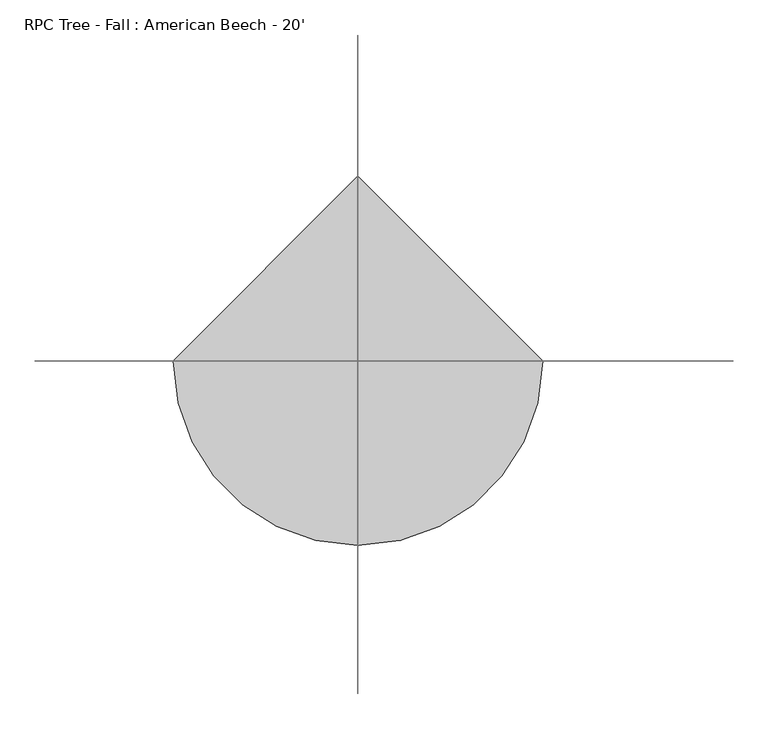
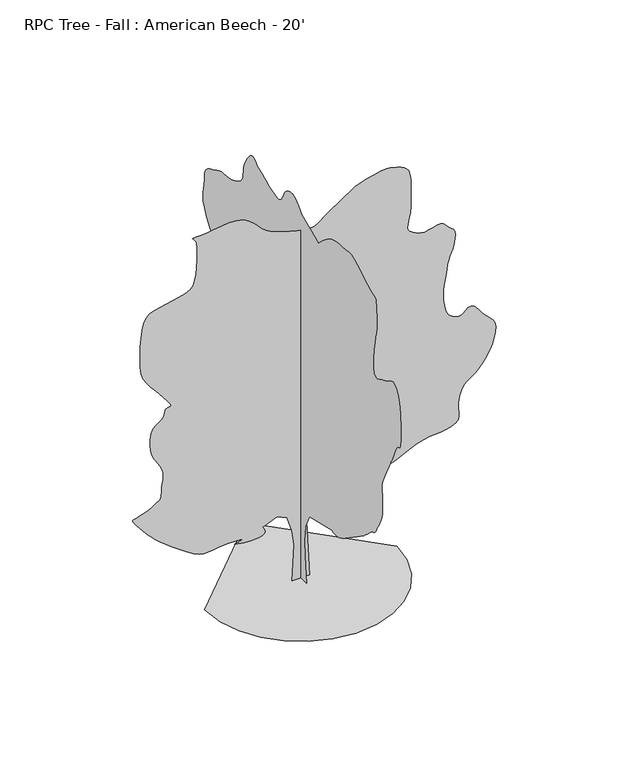
"""IFC4 building model written with IfcOpenShell, lengths in millimetres: geographic element geometry, RPC Tree - Fall : American Beech - 20'."""

from ifc_helpers import new_model, si_unit, origin, place, context, project, spatial, triangles, source, transform, mapped, element, save


def rpc_tree_fall_american_beech_20_7ed35302(model_context):
    return source(origin(), model_context, "Body", "Tessellation", [
        triangles([(0.0003461, 47.8998015, 0.0), (0.0003461, -52.4491741, 0.0), (0.0003461, -39.0692677, 147.1785164), (0.0003461, -35.7244046, 230.8023728), (0.0003461, -42.4141353, 314.4262293), (0.0003461, -82.5537637, 391.3603415), (0.0003461, -286.5960421, 441.5346408), (0.0003461, -297.4800798, 437.3999004), (0.0003461, -309.1526776, 434.2599395), (0.0003461, -322.4059021, 433.1087016), (0.0003461, -338.0291854, 434.9427103), (0.0003461, -356.8111058, 440.7550009), (0.0003461, -379.5428578, 451.5403527), (0.0003461, -407.0147638, 468.2944536), (0.0003461, -517.3983968, 545.2285658), (0.0003461, -533.0021682, 556.1997348), (0.0003461, -548.4298602, 566.6437194), (0.0003461, -563.9162696, 577.2637107), (0.0003461, -579.6951393, 588.7620641), (0.0003461, -596.0002851, 601.8392455), (0.0003461, -613.0664309, 617.1985188), (0.0003461, -631.1273924, 635.5421665), (0.0003461, -646.779126, 650.3066723), (0.0003461, -657.6329693, 656.9973249), (0.0003461, -665.4445564, 659.4154186), (0.0003461, -671.9689402, 661.365881), (0.0003461, -678.9609552, 666.6518229), (0.0003461, -688.1763084, 679.0756285), (0.0003461, -701.3708519, 702.4421528), (0.0003461, -715.7362541, 729.1227917), (0.0003461, -727.4097422, 750.8313503), (0.0003461, -736.5664507, 770.3741982), (0.0003461, -743.3832584, 790.5616287), (0.0003461, -748.0354454, 814.2001568), (0.0003461, -750.6971289, 844.0999306), (0.0003461, -751.5460596, 883.0692816), (0.0003461, -749.8880939, 918.7111467), (0.0003461, -746.4752209, 940.9005627), (0.0003461, -743.6463964, 955.8269045), (0.0003461, -743.7442102, 969.7041824), (0.0003461, -749.1075457, 988.7288206), (0.0003461, -762.0780476, 1019.1148293), (0.0003461, -784.9956167, 1067.040901), (0.0003461, -808.0492241, 1113.6867456), (0.0003461, -821.9754089, 1140.7834929), (0.0003461, -829.9328447, 1155.4253317), (0.0003461, -835.081949, 1164.679854), (0.0003461, -840.5821947, 1175.6323105), (0.0003461, -849.5930546, 1195.3592314), (0.0003461, -865.2741468, 1230.94594), (0.0003461, -882.983967, 1263.376664), (0.0003461, -896.3616388, 1275.8049751), (0.0003461, -905.9984053, 1278.5164375), (0.0003461, -912.4703213, 1281.8146374), (0.0003461, -916.3730627, 1295.9941498), (0.0003461, -918.2844286, 1331.3496952), (0.0003461, -918.7911564, 1398.1935802), (0.0003461, -915.3773386, 1473.7498695), (0.0003461, -906.2295685, 1530.0057381), (0.0003461, -892.9922951, 1569.3440346), (0.0003461, -877.2890385, 1594.1739143), (0.0003461, -860.7686806, 1606.8865105), (0.0003461, -845.0680401, 1609.8914143), (0.0003461, -831.8246624, 1605.5797588), (0.0003461, -820.3467293, 1598.43223), (0.0003461, -808.8101515, 1591.4001011), (0.0003461, -797.1562843, 1584.6082191), (0.0003461, -785.3272099, 1578.1541073), (0.0003461, -773.263484, 1572.179908), (0.0003461, -760.9081335, 1566.7837257), (0.0003461, -748.2007696, 1562.0986919), (0.0003461, -733.7483088, 1555.2800674), (0.0003461, -717.3649338, 1546.4701401), (0.0003461, -700.8054794, 1540.238253), (0.0003461, -685.8267426, 1541.1450291), (0.0003461, -674.1826132, 1553.7598114), (0.0003461, -667.6288708, 1582.6346478), (0.0003461, -667.9213675, 1632.3385906), (0.0003461, -673.2757645, 1686.7987839), (0.0003461, -680.0340002, 1729.2575294), (0.0003461, -687.1433046, 1763.2884464), (0.0003461, -693.5503263, 1792.4654446), (0.0003461, -698.2025133, 1820.3622883), (0.0003461, -700.0454241, 1850.5350105), (0.0003461, -698.0264339, 1886.5572304), (0.0003461, -695.2279129, 1921.1216904), (0.0003461, -694.0668646, 1945.9691563), (0.0003461, -692.4969023, 1963.2691177), (0.0003461, -688.4696772, 1975.1817627), (0.0003461, -679.9361864, 1983.8851559), (0.0003461, -664.8498253, 1991.5304741), (0.0003461, -641.1623903, 2000.287207), (0.0003461, -611.9542894, 2013.186565), (0.0003461, -581.9869689, 2030.1842194), (0.0003461, -551.7254076, 2048.8265408), (0.0003461, -521.640725, 2066.6421684), (0.0003461, -492.1996805, 2081.1773277), (0.0003461, -463.8699054, 2089.9874004), (0.0003461, -437.1198667, 2090.6007351), (0.0003461, -410.9841436, 2087.1692585), (0.0003461, -384.4972429, 2084.8489059), (0.0003461, -358.1277042, 2082.6975838), (0.0003461, -332.3431226, 2079.7904938), (0.0003461, -307.6120377, 2075.194408), (0.0003461, -284.40199, 2067.9579311), (0.0003461, -263.1815556, 2057.1476898), (0.0003461, -244.2822913, 2044.4438141), (0.0003461, -227.4890576, 2032.0867195), (0.0003461, -212.4516034, 2020.022921), (0.0003461, -198.8178971, 2008.1992241), (0.0003461, -186.2376512, 1996.5444122), (0.0003461, -174.3597061, 1985.005291), (0.0003461, -162.8329206, 1973.5282299), (0.0003461, -5.6196759, 2040.4256001), (0.0003461, 7.9941966, 2055.3518692), (0.0003461, 21.5788041, 2069.5581242), (0.0003461, 35.1049498, 2082.2885971), (0.0003461, 48.5432624, 2092.8321396), (0.0003461, 61.8645832, 2100.4508606), (0.0003461, 75.0396602, 2104.4068691), (0.0003461, 88.0391665, 2103.980151), (0.0003461, 100.5219802, 2100.8509815), (0.0003461, 112.1269949, 2096.9570332), (0.0003461, 122.7958931, 2091.9519608), (0.0003461, 132.4699938, 2085.4889832), (0.0003461, 141.090634, 2077.2124535), (0.0003461, 148.5991328, 2066.7665794), (0.0003461, 154.9385987, 2053.8050159), (0.0003461, 160.9846868, 2039.4298759), (0.0003461, 168.0842534, 2025.6414734), (0.0003461, 176.8809185, 2013.4355324), (0.0003461, 188.0174299, 2003.7987659), (0.0003461, 202.1383158, 1997.7268982), (0.0003461, 219.8872142, 1996.2333847), (0.0003461, 241.9077633, 2000.287207), (0.0003461, 265.8876586, 2007.941391), (0.0003461, 289.1661432, 2016.4758991), (0.0003461, 311.8587988, 2025.7392872), (0.0003461, 334.0837867, 2035.5894127), (0.0003461, 355.9576695, 2045.8751221), (0.0003461, 377.5977004, 2056.4542728), (0.0003461, 399.1204419, 2067.1844318), (0.0003461, 409.1750244, 2076.3234089), (0.0003461, 419.3460969, 2084.3777138), (0.0003461, 429.7518208, 2090.2718307), (0.0003461, 440.5078503, 2092.9120766), (0.0003461, 451.7332552, 2091.2230808), (0.0003461, 463.5427451, 2084.1287464), (0.0003461, 476.0545541, 2070.5271057), (0.0003461, 488.3129628, 2053.8760872), (0.0003461, 499.1667698, 2038.0341763), (0.0003461, 508.4408403, 2022.6099724), (0.0003461, 515.9600035, 2007.1769028), (0.0003461, 521.5482525, 1991.3438576), (0.0003461, 525.0295807, 1974.6839733), (0.0003461, 526.2288534, 1956.7972744), (0.0003461, 527.5259036, 1938.7682877), (0.0003461, 531.6900026, 1921.9129211), (0.0003461, 539.1309365, 1906.1598129), (0.0003461, 550.258564, 1891.4646343), (0.0003461, 565.4808907, 1877.7650345), (0.0003461, 585.2096283, 1864.9990986), (0.0003461, 609.8527462, 1853.1041851), (0.0003461, 636.1351536, 1844.2141754), (0.0003461, 660.7781988, 1839.2980511), (0.0003461, 684.192758, 1836.6043201), (0.0003461, 706.7884718, 1834.3817814), (0.0003461, 728.9743269, 1830.8702225), (0.0003461, 751.1602547, 1824.3182968), (0.0003461, 773.7559685, 1812.9657921), (0.0003461, 796.7224445, 1800.8753963), (0.0003461, 819.0443378, 1791.5942768), (0.0003461, 839.6700411, 1782.5975876), (0.0003461, 857.5460575, 1771.3872253), (0.0003461, 871.618091, 1755.4296238), (0.0003461, 880.8334442, 1732.2178139), (0.0003461, 884.1396378, 1699.2359608), (0.0003461, 886.3630486, 1665.3028576), (0.0003461, 891.2765568, 1638.6773026), (0.0003461, 896.2549593, 1616.0343533), (0.0003461, 898.6552488, 1594.0316265), (0.0003461, 895.8460453, 1569.3440346), (0.0003461, 885.1931345, 1538.6201832), (0.0003461, 864.0695692, 1498.5439957), (0.0003461, 837.9347546, 1458.3167999), (0.0003461, 814.3149027, 1427.3884552), (0.0003461, 793.679389, 1402.7898113), (0.0003461, 776.4959175, 1381.5159645), (0.0003461, 763.233791, 1360.5977646), (0.0003461, 754.3588966, 1337.0481846), (0.0003461, 750.341482, 1307.8800522), (0.0003461, 752.3017548, 1276.1071369), (0.0003461, 759.8786905, 1246.6189659), (0.0003461, 771.3183266, 1219.2289227), (0.0003461, 784.8640841, 1193.7768425), (0.0003461, 798.7600382, 1170.0849747), (0.0003461, 811.253171, 1147.96663), (0.0003461, 820.5858862, 1127.2529234), (0.0003461, 829.6252327, 1113.2422234), (0.0003461, 840.888862, 1107.7126917), (0.0003461, 852.0938467, 1105.2234541), (0.0003461, 860.9589306, 1100.333927), (0.0003461, 865.2012589, 1087.6123924), (0.0003461, 862.5387033, 1061.600172), (0.0003461, 850.6900806, 1016.8656933), (0.0003461, 834.365423, 966.4682608), (0.0003461, 819.2106068, 925.3697519), (0.0003461, 804.3482872, 891.0098579), (0.0003461, 788.9009743, 860.7953505), (0.0003461, 771.9913233, 832.1633045), (0.0003461, 752.7400274, 802.5364792), (0.0003461, 730.2714134, 769.3411943), (0.0003461, 707.7343443, 735.8818995), (0.0003461, 688.8253241, 706.8693535), (0.0003461, 673.4856354, 681.8359978), (0.0003461, 661.6556889, 660.3123842), (0.0003461, 653.2785839, 641.8326982), (0.0003461, 648.2957485, 625.9267651), (0.0003461, 646.6475933, 612.12768), (0.0003461, 648.0521587, 602.6580182), (0.0003461, 651.3290663, 598.2210071), (0.0003461, 655.0735325, 596.0660877), (0.0003461, 657.881864, 593.4426287), (0.0003461, 658.3503674, 587.6010158), (0.0003461, 655.0735325, 575.7915258), (0.0003461, 646.6475933, 555.2636364), (0.0003461, 639.63603, 533.604021), (0.0003461, 638.8848404, 518.790572), (0.0003461, 640.4156336, 508.6586323), (0.0003461, 640.2503094, 501.0416917), (0.0003461, 634.4086601, 493.7767645), (0.0003461, 618.912513, 484.6974132), (0.0003461, 589.7835134, 471.6397799), (0.0003461, 558.0399568, 458.2985521), (0.0003461, 534.8983824, 448.8777972), (0.0003461, 516.6720966, 441.9738218), (0.0003461, 499.674406, 436.1810795), (0.0003461, 480.2186168, 430.0958768), (0.0003461, 454.6198523, 422.3135756), (0.0003461, 419.1905105, 411.43041), (0.0003461, 383.6242584, 400.9953275), (0.0003461, 357.8885837, 394.7145335), (0.0003461, 338.706615, 391.4190225), (0.0003461, 322.8006091, 389.9361551), (0.0003461, 306.8954753, 389.0978342), (0.0003461, 287.7126346, 387.7323289), (0.0003461, 261.9769598, 384.6705972), (0.0003461, 231.872729, 379.7846672), (0.0003461, 201.767608, 373.8452405), (0.0003461, 171.6633772, 367.0292685), (0.0003461, 141.5582472, 359.5101053), (0.0003461, 111.4540164, 351.4646662), (0.0003461, 81.3493405, 343.0680493), (0.0003461, 51.2446691, 334.4962978), (47.6644825, 0.0001104, 0.0049238), (-45.9942311, 0.0001104, 0.0049238), (-35.9593671, 9.87e-05, 197.3572668), (-45.9942311, 9.42e-05, 277.6367053), (-72.7539531, 8.92e-05, 361.2605435), (-126.2736605, 8.75e-05, 388.0203564), (-203.2077817, 8.92e-05, 354.5708356), (-196.9465542, 8.98e-05, 345.9981757), (-191.8267904, 9.03e-05, 337.6024673), (-188.9891002, 9.09e-05, 329.5569918), (-189.5740754, 9.14e-05, 322.0378286), (-194.7231616, 9.2e-05, 315.2209846), (-205.5769685, 9.2e-05, 309.2824662), (-223.2769783, 9.25e-05, 304.3965181), (-244.0973644, 9.25e-05, 301.1685538), (-263.6900638, 9.25e-05, 299.8715036), (-282.2577168, 9.25e-05, 300.1835303), (-300.0066334, 9.25e-05, 301.7828513), (-317.1412162, 9.25e-05, 304.3476112), (-333.8659947, 9.2e-05, 307.5560091), (-350.3854079, 9.2e-05, 311.0862442), (-333.6508553, 9.2e-05, 315.3481207), (-319.7255424, 9.14e-05, 319.3752731), (-311.4160569, 9.14e-05, 322.9348306), (-311.5334189, 9.09e-05, 325.7921053), (-322.8850516, 9.09e-05, 327.713209), (-348.2793591, 9.09e-05, 328.4644349), (-390.524673, 9.09e-05, 327.8110228), (-435.0334024, 9.14e-05, 324.7395169), (-468.0739729, 9.14e-05, 320.0286853), (-493.7412289, 9.14e-05, 316.1375347), (-516.1315773, 9.14e-05, 315.5232553), (-539.3416068, 9.14e-05, 320.643001), (-567.466925, 9.09e-05, 333.9549065), (-604.6022673, 8.92e-05, 357.9152535), (-645.7754808, 8.75e-05, 387.0451252), (-683.3215176, 8.59e-05, 414.4192537), (-717.2973507, 8.42e-05, 440.3300632), (-747.7624969, 8.31e-05, 465.0718306), (-774.7765457, 8.14e-05, 488.9344002), (-798.3955256, 7.97e-05, 512.2128848), (-818.6798979, 7.86e-05, 535.1988728), (-837.1310972, 7.75e-05, 557.4327991), (-854.4701551, 7.58e-05, 577.91269), (-869.5858023, 7.47e-05, 596.1096534), (-881.3659698, 7.41e-05, 611.4982853), (-888.6993158, 7.36e-05, 623.5522007), (-890.4764603, 7.3e-05, 631.7443605), (-885.5789394, 7.25e-05, 635.5474714), (-874.5597719, 7.25e-05, 637.9558273), (-859.6779041, 7.25e-05, 642.11989), (-842.3966188, 7.19e-05, 647.7472355), (-824.1801435, 7.14e-05, 654.5445677), (-806.4898716, 7.08e-05, 662.2193172), (-790.7892311, 7.08e-05, 670.4789875), (-778.5405602, 7.02e-05, 679.0320992), (-768.9447069, 6.97e-05, 685.5262522), (-760.342761, 6.97e-05, 689.2129457), (-752.9116013, 6.91e-05, 692.1972839), (-746.8263622, 6.91e-05, 696.5853882), (-742.2631233, 6.86e-05, 704.4850513), (-739.3961472, 6.75e-05, 718.0014502), (-738.4012951, 6.63e-05, 739.2414328), (-737.0162779, 6.52e-05, 763.3680124), (-733.8762806, 6.36e-05, 784.8027506), (-730.5016319, 6.24e-05, 804.541226), (-728.415204, 6.13e-05, 823.577346), (-729.137035, 6.02e-05, 842.9060354), (-734.1883255, 5.91e-05, 863.5210562), (-745.0910757, 5.74e-05, 886.4190771), (-758.938995, 5.63e-05, 908.8520828), (-771.4997108, 5.52e-05, 928.6501476), (-782.3046473, 5.41e-05, 947.6836515), (-790.8870449, 5.3e-05, 967.8284248), (-796.7766563, 5.13e-05, 990.9602251), (-799.507667, 4.96e-05, 1018.9459442), (-798.6107014, 4.79e-05, 1053.6702782), (-792.5930454, 4.57e-05, 1085.9765911), (-781.6022919, 4.46e-05, 1107.7482273), (-767.6281448, 4.35e-05, 1122.3900661), (-752.658201, 4.29e-05, 1133.2803171), (-738.684054, 4.24e-05, 1143.8238596), (-727.6933004, 4.13e-05, 1157.4078415), (-721.6765892, 4.01e-05, 1177.4281311), (-715.3859848, 3.96e-05, 1194.5591349), (-704.9420002, 3.9e-05, 1200.9688454), (-694.3797815, 3.9e-05, 1202.3556793), (-687.7389805, 3.85e-05, 1204.3825905), (-689.0555426, 3.85e-05, 1212.7303368), (-702.367448, 3.68e-05, 1233.0795307), (-731.7107151, 3.46e-05, 1271.0931988), (-766.9942446, 3.23e-05, 1313.8007664), (-795.665387, 3.01e-05, 1347.3872337), (-818.0753563, 2.84e-05, 1376.2353275), (-834.5760933, 2.68e-05, 1404.7277744), (-845.5179399, 2.51e-05, 1437.2651779), (-851.251965, 2.23e-05, 1478.2215443), (-852.1293823, 1.9e-05, 1531.9971863), (-850.3353785, 1.56e-05, 1589.5599518), (-847.1954538, 1.28e-05, 1639.0506809), (-841.772529, 1.06e-05, 1680.5847736), (-833.1323587, 8.4e-06, 1714.2779205), (-820.3378635, 6.7e-06, 1740.2543873), (-802.4520367, 5.6e-06, 1758.6122784), (-778.5405602, 5e-06, 1769.4847252), (-748.4452314, 4.5e-06, 1776.1789387), (-714.3129398, 4.5e-06, 1782.4552998), (-678.6595928, 3.9e-06, 1789.1495132), (-644.0010252, 3.3e-06, 1797.0705414), (-612.8530718, 2.8e-06, 1807.0362122), (-587.7317127, 2.2e-06, 1819.8644989), (-571.1527465, 1.1e-06, 1836.3909611), (-561.4394949, -6e-07, 1860.7496487), (-554.8866972, -2.2e-06, 1894.0604061), (-550.966188, -4.5e-06, 1932.5808746), (-549.1526359, -7.2e-06, 1972.5681141), (-548.9179482, -9.5e-06, 2010.2706093), (-549.7375929, -1.11e-05, 2041.9457108), (-551.08355, -1.23e-05, 2063.841758), (-555.071606, -1.34e-05, 2077.6569031), (-562.1035895, -1.39e-05, 2087.8981384), (-569.0760201, -1.45e-05, 2095.0901413), (-572.8889414, -1.45e-05, 2099.7751751), (-570.4415254, -1.51e-05, 2102.4600403), (-558.6311634, -1.51e-05, 2103.6957207), (-534.3587714, -1.51e-05, 2103.9891621), (-500.0700213, -1.51e-05, 2106.238298), (-461.5691737, -1.56e-05, 2111.3589157), (-420.7853622, -1.56e-05, 2116.8885201), (-379.6513178, -1.56e-05, 2120.3644707), (-340.0970098, -1.56e-05, 2119.3421494), (-304.0533523, -1.56e-05, 2111.3589157), (-273.4512776, -1.45e-05, 2093.9522747), (-250.2127978, -1.28e-05, 2072.9185295), (-232.9413048, -1.17e-05, 2055.0940361), (-218.5963773, -1.11e-05, 2039.6164925), (-204.1341242, -1e-05, 2025.6058651), (-186.5123437, -9.5e-06, 2012.1819752), (-162.6880167, -8.4e-06, 1998.4557781), (-129.6180784, -7.8e-06, 1983.5651173), (-91.3021487, -6.7e-06, 1969.5810871), (-54.507833, -6.1e-06, 1958.9308651), (-20.3462917, -5.6e-06, 1951.2676701), (10.0704223, -5.6e-06, 1946.2358551), (35.6307035, -5.6e-06, 1943.4889297), (55.2225922, -5e-06, 1942.6620907), (67.7344738, -5.6e-06, 1943.4267242), (76.7453882, -5.6e-06, 1946.2181236), (86.5754205, -5.6e-06, 1951.4009468), (97.2246705, -6.1e-06, 1958.5218784), (108.6927841, -6.7e-06, 1967.1007153), (120.9805515, -7.2e-06, 1976.6841419), (134.0870916, -7.8e-06, 1986.7832348), (148.0132856, -8.4e-06, 1996.9445332), (281.8123406, -1.39e-05, 2087.2580612), (290.6276638, -1.39e-05, 2090.5473953), (313.8377114, -1.45e-05, 2098.8061935), (346.5849132, -1.51e-05, 2109.6431774), (384.0136242, -1.62e-05, 2120.648901), (421.2663285, -1.62e-05, 2129.4412422), (453.4872542, -1.67e-05, 2133.6017441), (475.8198664, -1.67e-05, 2130.7479939), (492.6219658, -1.62e-05, 2124.7294659), (510.7122497, -1.56e-05, 2119.8844128), (528.9198592, -1.56e-05, 2114.505962), (546.0731363, -1.51e-05, 2106.9138382), (561.003911, -1.45e-05, 2095.3924484), (572.5404525, -1.34e-05, 2078.261372), (579.5137914, -1.17e-05, 2053.8138817), (582.8582093, -1e-05, 2026.4238384), (584.5650819, -8.9e-06, 2001.0339638), (585.0424873, -7.2e-06, 1976.7464928), (584.7010838, -6.1e-06, 1952.698978), (583.9498941, -4.5e-06, 1928.0113861), (583.1995766, -2.8e-06, 1901.7948177), (582.8582093, -1.1e-06, 1873.1866802), (581.0828816, 6e-07, 1844.7030991), (576.8512359, 2.2e-06, 1819.4466465), (571.799037, 3.3e-06, 1797.346106), (567.5665192, 4.5e-06, 1778.3570034), (565.7920635, 5.6e-06, 1762.3994019), (568.1132518, 6.1e-06, 1749.4289726), (576.168465, 6.7e-06, 1739.3832195), (587.4419048, 7.2e-06, 1731.3911201), (598.3641669, 7.8e-06, 1724.5636299), (608.9939323, 7.8e-06, 1718.8472637), (619.38901, 8.4e-06, 1714.1889725), (629.6098978, 8.4e-06, 1710.5173943), (639.7124788, 8.9e-06, 1707.7882004), (649.7572872, 8.9e-06, 1705.9301743), (662.5713306, 8.9e-06, 1706.9881039), (679.774423, 8.4e-06, 1711.4952415), (699.6097675, 8.4e-06, 1717.1671337), (720.3234741, 7.8e-06, 1721.7366222), (740.1588913, 7.8e-06, 1722.901086), (757.361911, 8.4e-06, 1718.3939484), (770.1759544, 8.9e-06, 1705.9301743), (780.669718, 9.5e-06, 1691.9728867), (791.4551062, 1e-05, 1682.682756), (801.5968563, 1.06e-05, 1675.3929394), (810.1597057, 1.11e-05, 1667.3919743), (816.2057756, 1.17e-05, 1656.0038612), (818.799876, 1.28e-05, 1638.526149), (817.0058722, 1.45e-05, 1612.2739723), (811.9634474, 1.62e-05, 1584.4304684), (805.7520533, 1.73e-05, 1562.3831223), (798.837359, 1.84e-05, 1543.7319351), (791.6888855, 1.95e-05, 1526.067461), (784.775136, 2.06e-05, 1506.9984215), (778.5627972, 2.23e-05, 1484.1333927), (773.5213171, 2.4e-05, 1455.0630741), (768.918037, 2.56e-05, 1423.9568333), (764.139695, 2.73e-05, 1395.828899), (759.8289116, 2.9e-05, 1369.5767223), (756.6302696, 3.07e-05, 1344.0801682), (755.1874071, 3.18e-05, 1318.2369781), (756.1430901, 3.34e-05, 1290.9357376), (760.1409565, 3.51e-05, 1261.0564568), (766.4902056, 3.68e-05, 1233.7552162), (774.0671413, 3.79e-05, 1213.8949459), (782.8727085, 3.9e-05, 1199.8842459), (792.9077065, 3.96e-05, 1190.1407999), (804.1714085, 4.01e-05, 1183.0910122), (816.6644686, 4.01e-05, 1177.1436281), (830.3853607, 4.07e-05, 1170.7427834), (844.3986769, 4.07e-05, 1169.8716156), (858.1203684, 4.01e-05, 1178.1304138), (872.0750399, 3.96e-05, 1190.3097576), (886.7915108, 3.9e-05, 1201.2088743), (902.7980192, 3.85e-05, 1205.6005394), (920.6135742, 3.9e-05, 1198.301857), (940.7672132, 4.07e-05, 1174.0854572), (962.4499741, 4.24e-05, 1144.4906067), (983.5459248, 4.35e-05, 1122.4345402), (1002.6417068, 4.46e-05, 1104.8322716), (1018.3592068, 4.57e-05, 1088.581374), (1029.2672619, 4.68e-05, 1070.5701914), (1033.9789656, 4.79e-05, 1047.6962242), (1031.080814, 5.02e-05, 1016.874559), (1023.4531546, 5.18e-05, 983.7148825), (1014.7231642, 5.35e-05, 955.1778889), (1004.57967, 5.52e-05, 930.1614653), (992.7381689, 5.63e-05, 907.5363928), (978.905365, 5.74e-05, 886.1950356), (962.7966825, 5.91e-05, 865.0332458), (944.1098871, 6.02e-05, 842.9344494), (924.8540857, 6.13e-05, 823.9765223), (907.1718801, 6.24e-05, 810.8699821), (891.0098579, 6.3e-05, 800.4544842), (876.3173681, 6.36e-05, 789.5712822), (863.0250109, 6.41e-05, 775.0601767), (851.0785744, 6.58e-05, 753.7623487), (840.4203587, 6.75e-05, 722.5166542), (834.6765232, 6.97e-05, 688.013673), (835.0179268, 7.14e-05, 658.6597235), (837.6991585, 7.25e-05, 633.8699575), (838.9766241, 7.41e-05, 613.0593092), (835.1050581, 7.53e-05, 595.642022), (822.3398489, 7.58e-05, 581.0331027), (796.9358036, 7.64e-05, 568.6484299), (766.41194, 7.69e-05, 560.4073631), (739.1062666, 7.75e-05, 556.789161), (712.5020765, 7.75e-05, 555.0440277), (684.0842617, 7.75e-05, 552.420605), (651.33706, 7.8e-05, 546.1700418), (611.7436192, 7.86e-05, 533.5408708), (562.7881408, 8.03e-05, 511.7834779), (509.4836546, 8.14e-05, 486.7598963), (459.1048619, 8.25e-05, 466.0079653), (412.5283444, 8.36e-05, 449.2929608), (370.634172, 8.47e-05, 436.3811036), (334.2980541, 8.53e-05, 427.0386143), (304.3982803, 8.53e-05, 421.0307324), (281.8123406, 8.59e-05, 418.1245872), (141.3235504, 8.59e-05, 414.7801692), (37.6296231, 8.7e-05, 398.0553906), (30.9398924, 9.2e-05, 307.7409179), (-508.8151271, 0.0, 0.0042102), (-495.3636589, -116.587106, 0.0042102), (-457.0548417, -223.6530272, 0.0042102), (-396.9548038, -318.1315627, 0.0042102), (-318.1315627, -396.9548038, 0.0042102), (-223.6530272, -457.0548417, 0.0042102), (-116.587106, -495.3636589, 0.0042102), (2.22e-05, -508.8151271, 0.0042102), (116.587106, -495.3636589, 0.0042102), (223.6530272, -457.0548417, 0.0042102), (318.1315627, -396.9548038, 0.0042102), (396.9548038, -318.1315627, 0.0042102), (457.0548417, -223.6530272, 0.0042102), (495.3636589, -116.587106, 0.0042102), (508.8151271, 4.46e-05, 0.0042102), (-6.67e-05, 508.8151271, 0.0042102)], [[1, 2, 3], [254, 1, 3], [254, 3, 4], [254, 4, 5], [254, 5, 6], [53, 54, 55], [52, 53, 55], [201, 202, 203], [201, 203, 204], [200, 201, 204], [222, 223, 224], [52, 55, 56], [200, 204, 205], [199, 200, 205], [253, 254, 6], [221, 222, 224], [221, 224, 225], [229, 230, 231], [229, 231, 232], [228, 229, 232], [228, 232, 233], [227, 228, 233], [252, 253, 6], [221, 225, 226], [220, 221, 226], [199, 205, 206], [198, 199, 206], [62, 63, 64], [61, 62, 64], [61, 64, 65], [60, 61, 65], [60, 65, 66], [59, 60, 66], [59, 66, 67], [59, 67, 68], [58, 59, 68], [58, 68, 69], [58, 69, 70], [57, 58, 70], [57, 70, 71], [57, 71, 72], [57, 72, 73], [57, 73, 74], [56, 57, 74], [52, 56, 74], [51, 52, 74], [50, 51, 74], [50, 74, 75], [49, 50, 75], [48, 49, 75], [47, 48, 75], [46, 47, 75], [45, 46, 75], [44, 45, 75], [43, 44, 75], [42, 43, 75], [42, 75, 76], [41, 42, 76], [227, 233, 234], [226, 227, 234], [220, 226, 234], [219, 220, 234], [219, 234, 235], [219, 235, 236], [219, 236, 237], [218, 219, 237], [218, 237, 238], [218, 238, 239], [218, 239, 240], [217, 218, 240], [217, 240, 241], [217, 241, 242], [217, 242, 243], [217, 243, 244], [217, 244, 245], [217, 245, 246], [216, 217, 246], [216, 246, 247], [215, 216, 247], [215, 247, 248], [251, 252, 6], [88, 89, 90], [88, 90, 91], [87, 88, 91], [87, 91, 92], [86, 87, 92], [86, 92, 93], [85, 86, 93], [84, 85, 93], [84, 93, 94], [83, 84, 94], [82, 83, 94], [81, 82, 94], [81, 94, 95], [80, 81, 95], [80, 95, 96], [80, 96, 97], [80, 97, 98], [80, 98, 99], [80, 99, 100], [80, 100, 101], [80, 101, 102], [80, 102, 103], [80, 103, 104], [80, 104, 105], [80, 105, 106], [80, 106, 107], [80, 107, 108], [80, 108, 109], [80, 109, 110], [80, 110, 111], [80, 111, 112], [79, 80, 112], [79, 112, 113], [78, 79, 113], [77, 78, 113], [76, 77, 113], [41, 76, 113], [40, 41, 113], [40, 113, 114], [39, 40, 114], [198, 206, 207], [197, 198, 207], [196, 197, 207], [196, 207, 208], [195, 196, 208], [195, 208, 209], [195, 209, 210], [195, 210, 211], [194, 195, 211], [194, 211, 212], [194, 212, 213], [193, 194, 213], [193, 213, 214], [214, 215, 248], [193, 214, 248], [193, 248, 249], [192, 193, 249], [192, 249, 250], [192, 250, 251], [192, 251, 6], [192, 6, 7], [191, 192, 7], [190, 191, 7], [189, 190, 7], [38, 39, 114], [37, 38, 114], [36, 37, 114], [35, 36, 114], [34, 35, 114], [33, 34, 114], [32, 33, 114], [31, 32, 114], [30, 31, 114], [29, 30, 114], [28, 29, 114], [27, 28, 114], [26, 27, 114], [25, 26, 114], [24, 25, 114], [23, 24, 114], [22, 23, 114], [21, 22, 114], [20, 21, 114], [19, 20, 114], [18, 19, 114], [17, 18, 114], [16, 17, 114], [15, 16, 114], [14, 15, 114], [13, 14, 114], [12, 13, 114], [11, 12, 114], [10, 11, 114], [9, 10, 114], [8, 9, 114], [7, 8, 114], [189, 7, 114], [188, 189, 114], [188, 114, 115], [188, 115, 116], [188, 116, 117], [188, 117, 118], [188, 118, 119], [188, 119, 120], [188, 120, 121], [146, 147, 148], [145, 146, 148], [144, 145, 148], [144, 148, 149], [143, 144, 149], [143, 149, 150], [142, 143, 150], [142, 150, 151], [142, 151, 152], [141, 142, 152], [141, 152, 153], [141, 153, 154], [141, 154, 155], [141, 155, 156], [140, 141, 156], [140, 156, 157], [139, 140, 157], [138, 139, 157], [138, 157, 158], [137, 138, 158], [137, 158, 159], [136, 137, 159], [135, 136, 159], [135, 159, 160], [134, 135, 160], [134, 160, 161], [174, 175, 176], [173, 174, 176], [173, 176, 177], [172, 173, 177], [171, 172, 177], [171, 177, 178], [170, 171, 178], [170, 178, 179], [169, 170, 179], [168, 169, 179], [167, 168, 179], [166, 167, 179], [165, 166, 179], [165, 179, 180], [165, 180, 181], [165, 181, 182], [165, 182, 183], [165, 183, 184], [165, 184, 185], [165, 185, 186], [165, 186, 187], [164, 165, 187], [164, 187, 188], [163, 164, 188], [162, 163, 188], [161, 162, 188], [134, 161, 188], [133, 134, 188], [132, 133, 188], [125, 126, 127], [124, 125, 127], [124, 127, 128], [123, 124, 128], [122, 123, 128], [121, 122, 128], [121, 128, 129], [121, 129, 130], [121, 130, 131], [188, 121, 131], [132, 188, 131], [274, 275, 276], [531, 255, 256], [531, 256, 257], [531, 257, 258], [531, 258, 259], [530, 531, 259], [376, 377, 378], [376, 378, 379], [375, 376, 379], [273, 274, 276], [273, 276, 277], [375, 379, 380], [374, 375, 380], [273, 277, 278], [272, 273, 278], [301, 302, 303], [301, 303, 304], [300, 301, 304], [300, 304, 305], [299, 300, 305], [299, 305, 306], [298, 299, 306], [298, 306, 307], [297, 298, 307], [297, 307, 308], [271, 272, 278], [296, 297, 308], [296, 308, 309], [373, 374, 380], [373, 380, 381], [372, 373, 381], [295, 296, 309], [295, 309, 310], [294, 295, 310], [294, 310, 311], [294, 311, 312], [294, 312, 313], [293, 294, 313], [293, 313, 314], [292, 293, 314], [271, 278, 279], [291, 292, 314], [530, 259, 260], [372, 381, 382], [371, 372, 382], [291, 314, 315], [290, 291, 315], [371, 382, 383], [370, 371, 383], [370, 383, 384], [369, 370, 384], [369, 384, 385], [369, 385, 386], [369, 386, 387], [369, 387, 388], [369, 388, 389], [369, 389, 390], [368, 369, 390], [368, 390, 391], [367, 368, 391], [367, 391, 392], [367, 392, 393], [366, 367, 393], [366, 393, 394], [270, 271, 279], [366, 394, 395], [338, 339, 340], [338, 340, 341], [289, 290, 315], [483, 484, 485], [483, 485, 486], [482, 483, 486], [481, 482, 486], [481, 486, 487], [480, 481, 487], [288, 289, 315], [287, 288, 315], [286, 287, 315], [285, 286, 315], [284, 285, 315], [283, 284, 315], [282, 283, 315], [282, 315, 316], [281, 282, 316], [281, 316, 317], [281, 317, 318], [281, 318, 319], [281, 319, 320], [280, 281, 320], [280, 320, 321], [279, 280, 321], [279, 321, 322], [480, 487, 488], [264, 265, 266], [263, 264, 266], [263, 266, 267], [262, 263, 267], [262, 267, 268], [261, 262, 268], [261, 268, 269], [261, 269, 270], [261, 270, 279], [261, 279, 322], [260, 261, 322], [530, 260, 322], [530, 322, 323], [529, 530, 323], [529, 323, 324], [366, 395, 396], [365, 366, 396], [337, 338, 341], [337, 341, 342], [529, 324, 325], [528, 529, 325], [527, 528, 325], [526, 527, 325], [525, 526, 325], [524, 525, 325], [523, 524, 325], [522, 523, 325], [521, 522, 325], [521, 325, 326], [521, 326, 327], [521, 327, 328], [521, 328, 329], [521, 329, 330], [521, 330, 331], [521, 331, 332], [521, 332, 333], [521, 333, 334], [521, 334, 335], [521, 335, 336], [521, 336, 337], [521, 337, 342], [520, 521, 342], [520, 342, 343], [519, 520, 343], [518, 519, 343], [518, 343, 344], [517, 518, 344], [449, 450, 451], [448, 449, 451], [448, 451, 452], [447, 448, 452], [446, 447, 452], [446, 452, 453], [516, 517, 344], [515, 516, 344], [514, 515, 344], [513, 514, 344], [512, 513, 344], [511, 512, 344], [510, 511, 344], [509, 510, 344], [508, 509, 344], [507, 508, 344], [506, 507, 344], [505, 506, 344], [504, 505, 344], [503, 504, 344], [502, 503, 344], [501, 502, 344], [500, 501, 344], [499, 500, 344], [498, 499, 344], [497, 498, 344], [496, 497, 344], [495, 496, 344], [494, 495, 344], [493, 494, 344], [492, 493, 344], [491, 492, 344], [490, 491, 344], [489, 490, 344], [488, 489, 344], [480, 488, 344], [479, 480, 344], [478, 479, 344], [477, 478, 344], [476, 477, 344], [475, 476, 344], [474, 475, 344], [473, 474, 344], [472, 473, 344], [471, 472, 344], [470, 471, 344], [469, 470, 344], [468, 469, 344], [467, 468, 344], [466, 467, 344], [465, 466, 344], [464, 465, 344], [463, 464, 344], [463, 344, 345], [462, 463, 345], [462, 345, 346], [461, 462, 346], [460, 461, 346], [459, 460, 346], [458, 459, 346], [457, 458, 346], [456, 457, 346], [455, 456, 346], [454, 455, 346], [453, 454, 346], [446, 453, 346], [445, 446, 346], [444, 445, 346], [443, 444, 346], [442, 443, 346], [441, 442, 346], [440, 441, 346], [439, 440, 346], [438, 439, 346], [437, 438, 346], [436, 437, 346], [435, 436, 346], [435, 346, 347], [435, 347, 348], [435, 348, 349], [435, 349, 350], [435, 350, 351], [435, 351, 352], [435, 352, 353], [435, 353, 354], [435, 354, 355], [435, 355, 356], [435, 356, 357], [435, 357, 358], [435, 358, 359], [435, 359, 360], [435, 360, 361], [435, 361, 362], [435, 362, 363], [435, 363, 364], [435, 364, 365], [435, 365, 396], [435, 396, 397], [435, 397, 398], [435, 398, 399], [435, 399, 400], [435, 400, 401], [435, 401, 402], [435, 402, 403], [435, 403, 404], [435, 404, 405], [435, 405, 406], [435, 406, 407], [435, 407, 408], [435, 408, 409], [434, 435, 409], [433, 434, 409], [432, 433, 409], [431, 432, 409], [430, 431, 409], [429, 430, 409], [429, 409, 410], [429, 410, 411], [429, 411, 412], [428, 429, 412], [428, 412, 413], [427, 428, 413], [426, 427, 413], [426, 413, 414], [425, 426, 414], [425, 414, 415], [425, 415, 416], [425, 416, 417], [424, 425, 417], [424, 417, 418], [423, 424, 418], [423, 418, 419], [422, 423, 419], [422, 419, 420], [421, 422, 420], [546, 547, 532], [545, 546, 532], [545, 532, 533], [544, 545, 533], [544, 533, 534], [544, 534, 535], [543, 544, 535], [542, 543, 535], [542, 535, 536], [542, 536, 537], [542, 537, 538], [542, 538, 539], [542, 539, 540], [542, 540, 541]], closed=False),
    ])


if __name__ == "__main__":
    model = new_model("IFC4")
    model_context = context("Model", 3, world=origin())
    ifc_project = project(units=[si_unit("LENGTHUNIT", "METRE", prefix="MILLI")], contexts=[model_context])
    site = spatial("IfcSite", under=ifc_project)
    building = spatial("IfcBuilding", under=site)
    placement = place(None, origin())
    rpc_tree_fall_american_beech_20_shape = rpc_tree_fall_american_beech_20_7ed35302(model_context)
    element("IfcGeographicElement", 1, ObjectType="RPC Tree - Fall : American Beech - 20'", at=placement, inside=building, context=model_context, shape_type="MappedRepresentation", body=[
        mapped(rpc_tree_fall_american_beech_20_shape, transform((0.0, 0.0, 0.0), x_axis=(1.0, 0.0, 0.0), y_axis=(0.0, 1.0, 0.0), z_axis=(0.0, 0.0, 1.0))),
    ])
    save(model, "model.ifc")

# Revit data of these elements
# Type "RPC Tree - Fall : American Beech - 20'"
#   built-in parameter 1005198 = "{2, 15},{39, RPC-16-G2VX-NFFX-5QM5-6000-ST1L-LVER-AU},{1, 0},{1, 0},{2, 13},{1, 8},{5, Color},{1, 0},{1, 0},{3, 0.8},{3, 0.8},{3, 0.8},{1, 8},{7, BBoxMin},{1, 0},{1, 0},{1, 0},{1, 0},{1, 0},{1, 8},{7, BBoxMax},{1, 0},{1, 0},{1, 0},{1, 0},{1, 0},{2, 11},{9, RPCTypeId},{1, 0},{1, 0},{39, RPC-16-G2VX-NFFX-5QM5-6000-ST1L-LVER-AU},{1, 6},{14, RPCPlantHeight},{1, 0},{1, 0},{2, 20},{2, 11},{7, keyword},{1, 0},{1, 0},{39, :RPCs:Fall Trees [General]:Geometry:RPC},{2, 11},{8, category},{1, 0},{1, 0},{20, Fall Trees [General]},{2, 11},{12, LocalizedUID},{1, 0},{1, 0},{21, American Beech [Fall]},{2, 14},{6, Height},{1, 0},{1, 0},{2, 20},{1, 2},{16, Cast Reflections},{1, 0},{1, 0},{1, 0},{1, 2},{12, Cast Shadows},{1, 0},{1, 0},{1, 1},{1, 2},{9, Lock View},{1, 0},{1, 0},{1, 0},{1, 4},{5, ViewC},{1, 0},{1, 0},{1, 0},{21, assetlibrary_base.fbx},{1, 5},"
#   built-in parameter 1005195 = "RPC-16-G2VX-NFFX-5QM5-6000-ST1L-LVER-AU"
#   Type Comments = "American Beech"
#   Assembly Code = "G2050500"
#   Height = 7' - 0"
#   Default Elevation = 0
